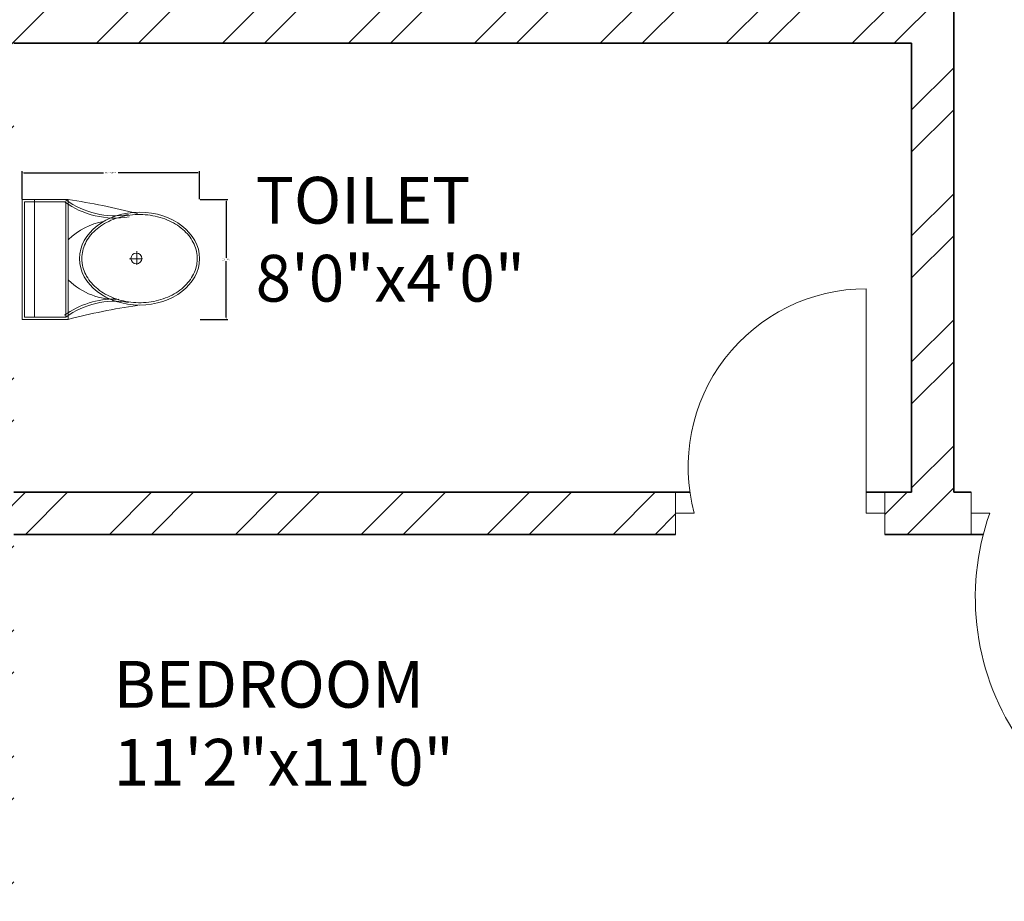
# Model space of a CAD drawing. Units: inches. Extents: x 1885 to 2748, y 783 to 2421.
# Tile 70 of 117: x 2022 to 2127, y 1979 to 2073. Entities that reach past the tile are written whole.
import ezdxf

# ---------------------------------------------------------------- set-up
doc = ezdxf.new("R2010")
doc.units = ezdxf.units.IN
for name, color, linetype, lineweight in [('A-ANNO-DIMS', 2, 'Continuous', 18), ('A-AREA-IDEN', 7, 'Continuous', 18), ('A-DOOR', 31, 'Continuous', 18), ('A-FLOR-FIXT', 8, 'Continuous', 18), ('A-WALL', 7, 'Continuous', 35)]:
    doc.layers.add(name, color=color, linetype=linetype, lineweight=lineweight)
doc.layers.add('A-WALL-PATT', color=85, linetype='Continuous', lineweight=13, true_color=0x58ba48)
doc.styles.get("Standard").update_dxf_attribs({"font": 'arial.ttf'})
doc.dimstyles.get("Standard").update_dxf_attribs({"dimtxt": 0.18, "dimasz": 0.18, "dimexe": 0.18, "dimexo": 0.0625, "dimgap": 0.09, "dimtad": 0, "dimtih": 1, "dimtoh": 1, "dimdec": 4, "dimzin": 0, "dimdsep": 46, "dimtxsty": 'Standard', "dimcen": 0.09, "dimadec": 0, "dimazin": 0, "dimtfac": 1, "dimtdec": 4, "dimtofl": 0, "dimtmove": 0, "dimatfit": 3, "dimfxl": 1, "dimtolj": 1, "dimtzin": 0, "dimarcsym": 0})

# ---------------------------------------------------------------- blocks, each defined once
blk = doc.blocks.new('A$C31115884')
for p, q in [((257.5, 466.4), (257.5, 523.2)), ((283.1, 497.7), (223.4, 497.7)), ((0, 200), (0, 0)), ((520, 200), (0, 200)), ((10, 190), (10, 10)), ((510, 190), (10, 190)), ((510, 10), (510, 190)), ((520, 0), (520, 200)), ((510, 54.5), (0, 54.5)), ((10, 10), (510, 10)), ((0, 0), (520, 0))]:
    blk.add_line(p, q)
blk.add_circle((255.6, 496.4), 23.6)
for centre, radius, start, end in [((2777.7, -204.6), 2807, 165.4549, 171.7133), ((3237, 905), 2807, 188.2867, 194.5451), ((-294.5, 403.3), 364.7, 324.2091, 9.3499), ((-294.5, 403.3), 374.7, 324.2091, 9.3499), ((805.8, 403.3), 364.7, 170.6501, 215.7909), ((139.5, 406.2), 293.5, 315.8436, 2.6563), ((805.8, 403.3), 374.7, 179.2036, 215.7909), ((383.6, 406.2), 293.5, 190.2774, 224.1564)]:
    blk.add_arc(centre, radius, start, end)
blk.add_ellipse((256.2, 509.9), major_axis=(0, -260.7), ratio=0.772727)
blk.add_open_spline([(256.2, 259.2), (263.1, 259.2), (270, 259.7), (287.8, 262.3), (298.7, 265.1), (319.9, 273.1), (330.2, 278.4), (350.1, 291.1), (359.7, 298.7), (377.7, 315.9), (386.2, 325.5), (401.7, 346.6), (408.8, 358.1), (421.3, 382.5), (426.8, 395.5), (435.9, 422.4), (439.5, 436.4), (444.8, 465.1), (446.5, 479.7), (447.9, 509.2), (447.6, 524), (445, 553.3), (442.7, 567.8), (436.3, 596), (432.1, 609.7), (421.9, 636), (416, 648.6), (402.5, 672.1), (395, 683), (378.6, 703), (369.8, 712.1), (351.1, 728), (341.3, 734.8), (320.9, 746.2), (310.4, 750.7), (288.9, 757.3), (278, 759.4), (256, 761), (245, 760.6), (223.1, 757.2), (212.3, 754.3), (191.1, 746.1), (180.8, 740.7), (160.9, 727.8), (151.4, 720.1), (133.5, 702.7), (125.1, 693), (109.6, 671.7), (102.6, 660.2), (90.2, 635.7), (84.9, 622.7), (76, 595.6), (72.4, 581.6), (67.2, 552.9), (65.6, 538.2), (64.4, 508.8), (64.8, 494), (67.5, 464.7), (69.9, 450.2), (76.6, 422), (80.8, 408.3), (91.1, 382.2), (97.2, 369.7), (110.8, 346.3), (118.4, 335.4), (134.8, 315.6), (143.7, 306.7), (162.4, 290.9), (172.3, 284.2), (192.8, 273), (203.3, 268.6), (224.8, 262.2), (235.8, 260.2), (249.9, 259.3), (253, 259.2), (256.2, 259.2)], degree=3, knots=[0, 0, 0, 0, 0.110105, 0.110105, 0.285049, 0.285049, 0.459994, 0.459994, 0.634938, 0.634938, 0.809882, 0.809882, 0.984827, 0.984827, 1.159771, 1.159771, 1.334715, 1.334715, 1.50966, 1.50966, 1.684604, 1.684604, 1.859549, 1.859549, 2.034493, 2.034493, 2.209437, 2.209437, 2.384382, 2.384382, 2.559326, 2.559326, 2.73427, 2.73427, 2.909215, 2.909215, 3.084159, 3.084159, 3.259103, 3.259103, 3.434048, 3.434048, 3.608992, 3.608992, 3.783936, 3.783936, 3.958881, 3.958881, 4.133825, 4.133825, 4.30877, 4.30877, 4.483714, 4.483714, 4.658658, 4.658658, 4.833603, 4.833603, 5.008547, 5.008547, 5.183491, 5.183491, 5.358436, 5.358436, 5.53338, 5.53338, 5.708324, 5.708324, 5.883269, 5.883269, 6.058213, 6.058213, 6.233158, 6.233158, 6.283185, 6.283185, 6.283185, 6.283185])
blk = doc.blocks.new('*D29')
at = {"layer": 'A-ANNO-DIMS', "color": 0, "lineweight": -2, "transparency": 16777216}
for p, q in [((2022.15, 2053.85), (2022.15, 2056.82)), ((2022.33, 2056.64), (2030.86, 2056.64)), ((2040.95, 2056.64), (2032.42, 2056.64)), ((2041.13, 2053.85), (2041.13, 2056.82))]:
    blk.add_line(p, q, dxfattribs=at)
at = {"layer": 'A-ANNO-DIMS', "color": 0, "transparency": 16777216}
for points in [[(2022.33, 2056.67), (2022.33, 2056.61), (2022.15, 2056.64)], [(2040.95, 2056.67), (2040.95, 2056.61), (2041.13, 2056.64)]]:
    blk.add_solid(points, dxfattribs=at)
at = {"layer": 'Defpoints', "color": 0, "transparency": 16777216}
for p in [(2041.13, 2056.64), (2022.15, 2053.79), (2041.13, 2053.79)]:
    blk.add_point(p, dxfattribs=at)
at = {"layer": 'A-ANNO-DIMS', "color": 0, "transparency": 16777216, "insert": (2031.64, 2056.64), "char_height": 0.18, "attachment_point": 5}
blk.add_mtext('\\A1;WC 19 TYP.', dxfattribs=at)
blk = doc.blocks.new('*D30')
at = {"layer": 'A-ANNO-DIMS', "color": 0, "lineweight": -2, "transparency": 16777216}
for p, q in [((2041.19, 2053.79), (2044.15, 2053.79)), ((2043.97, 2053.61), (2043.97, 2047.57)), ((2043.97, 2041.17), (2043.97, 2047.21)), ((2041.19, 2040.99), (2044.15, 2040.99))]:
    blk.add_line(p, q, dxfattribs=at)
at = {"layer": 'A-ANNO-DIMS', "color": 0, "transparency": 16777216}
for points in [[(2043.94, 2053.61), (2044, 2053.61), (2043.97, 2053.79)], [(2043.94, 2041.17), (2044, 2041.17), (2043.97, 2040.99)]]:
    blk.add_solid(points, dxfattribs=at)
at = {"layer": 'Defpoints', "color": 0, "transparency": 16777216}
for p in [(2041.13, 2053.79), (2041.13, 2040.99), (2043.97, 2040.99)]:
    blk.add_point(p, dxfattribs=at)
at = {"layer": 'A-ANNO-DIMS', "color": 0, "transparency": 16777216, "insert": (2043.97, 2047.39), "char_height": 0.18, "attachment_point": 5}
blk.add_mtext('\\A1;13 TYP.', dxfattribs=at)

msp = doc.modelspace()

# ---------------------------------------------------------------- hatches: boundary and pattern name
at = {"layer": 'A-WALL-PATT'}
h = msp.add_hatch(dxfattribs=at)
h.set_pattern_fill('ANSI32', color=256)
h.paths.add_polyline_path([(2007.77, 2318.01), (1980.77, 2318.01), (1980.77, 2281.22), (1985.27, 2281.22), (1985.27, 2313.51), (2007.77, 2313.51), (2007.77, 2315.76)])
h.paths.add_polyline_path([(2094.32, 2318.01), (2067.77, 2318.01), (2067.77, 2313.51), (2094.32, 2313.51), (2094.32, 2315.76)])
h.paths.add_polyline_path([(2131.37, 2315.76), (2131.37, 2318.01), (2131.19, 2318.01), (2112.61, 2318.01), (2112.61, 2313.51), (2117.27, 2313.51), (2117.27, 2255.2), (2121.77, 2255.2), (2121.77, 2313.51), (2131.37, 2313.51)])
h.paths.add_polyline_path([(2190.51, 2318.01), (2155.37, 2318.01), (2155.37, 2313.51), (2169.77, 2313.51), (2169.77, 2229.51), (2121.77, 2229.51), (2121.77, 2233.45), (2119.52, 2233.45), (2117.27, 2233.45), (2117.27, 2201.1), (2121.77, 2201.1), (2121.77, 2225.01), (2169.77, 2225.01), (2169.77, 2165.01), (2306.27, 2165.01), (2306.27, 2066.01), (2310.77, 2066.01), (2344.27, 2066.01), (2486.27, 2066.01), (2486.27, 1886.01), (2483.02, 1886.01), (2483.02, 1881.51), (2486.27, 1881.51), (2486.27, 1880.68), (2490.77, 1880.68), (2490.77, 2070.51), (2344.27, 2070.51), (2310.77, 2070.51), (2310.77, 2165.01), (2310.77, 2173.64), (2308.52, 2173.64), (2306.27, 2173.64), (2306.27, 2169.51), (2174.27, 2169.51), (2174.27, 2313.51), (2190.51, 2313.51), (2190.51, 2315.76)])
h.paths.add_polyline_path([(1985.27, 2221.22), (1980.77, 2221.22), (1980.77, 2165.01), (1992.77, 2165.01), (1992.77, 2141.93), (1997.27, 2141.93), (1997.27, 2165.01), (2117.27, 2165.01), (2117.27, 2163.13), (2121.77, 2163.13), (2121.77, 2172.73), (2119.52, 2172.73), (2117.27, 2172.73), (2117.27, 2169.51), (1985.27, 2169.51)])
h.paths.add_polyline_path([(1997.27, 2105.93), (1992.77, 2105.93), (1992.77, 2070.51), (2016.77, 2070.51), (2016.77, 2059.12), (2019.02, 2059.12), (2021.27, 2059.12), (2021.27, 2070.51), (2117.27, 2070.51), (2117.27, 2022.51), (2114.42, 2022.51), (2114.42, 2018.01), (2123.63, 2018.01), (2123.63, 2020.26), (2123.63, 2022.51), (2121.77, 2022.51), (2121.77, 2142.59), (2119.52, 2142.59), (2117.27, 2142.59), (2117.27, 2075.01), (1997.27, 2075.01)])
h.paths.add_polyline_path([(2092.03, 2020.26), (2092.03, 2022.51), (2021.27, 2022.51), (2021.27, 2035.12), (2016.77, 2035.12), (2016.77, 2018.01), (2016.77, 1978.78), (2021.27, 1978.78), (2021.27, 2018.01), (2092.03, 2018.01)])
h.paths.add_polyline_path([(2260.94, 2022.51), (2153.1, 2022.51), (2153.1, 2020.26), (2153.1, 2018.01), (2155.27, 2018.01), (2155.27, 1886.01), (2107.63, 1886.01), (2107.63, 1881.51), (2182.91, 1881.51), (2182.91, 1883.76), (2182.91, 1886.01), (2159.77, 1886.01), (2159.77, 2018.01), (2260.94, 2018.01), (2260.94, 2020.26)])
h.paths.add_polyline_path([(2047.63, 1883.76), (2047.63, 1886.01), (2021.27, 1886.01), (2021.27, 1918.78), (2019.02, 1918.78), (2016.77, 1918.78), (2016.77, 1881.51), (2047.63, 1881.51)])
h.paths.add_polyline_path([(2306.36, 1883.76), (2306.36, 1886.01), (2296.27, 1886.01), (2296.27, 1982.01), (2316.54, 1982.01), (2316.54, 1984.26), (2316.54, 1986.51), (2296.27, 1986.51), (2296.27, 2022.51), (2289.28, 2022.51), (2289.28, 2018.01), (2291.77, 2018.01), (2291.77, 1886.01), (2242.91, 1886.01), (2242.91, 1881.51), (2306.36, 1881.51)], flags=17)
h.paths.add_polyline_path([(1985.27, 1843.01), (2021.6, 1843.01), (2021.53, 1845.44), (2021.48, 1847.51), (1980.77, 1847.51), (1980.77, 1809.45), (1985.27, 1809.45)])
h.paths.add_polyline_path([(2131.48, 1845.26), (2131.48, 1847.51), (2081.53, 1847.51), (2081.53, 1843.01), (2117.27, 1843.01), (2117.27, 1784.15), (2119.52, 1784.15), (2121.77, 1784.15), (2121.77, 1843.01), (2131.48, 1843.01)])
h.paths.add_polyline_path([(2203.89, 1847.51), (2155.48, 1847.51), (2155.48, 1843.01), (2169.77, 1843.01), (2169.77, 1759.01), (2121.77, 1759.01), (2121.77, 1761.46), (2117.27, 1761.46), (2117.27, 1730.43), (2121.77, 1730.43), (2121.77, 1754.51), (2177.42, 1754.51), (2177.42, 1756.76), (2177.42, 1759.01), (2174.27, 1759.01), (2174.27, 1843.01), (2203.89, 1843.01)])
h.paths.add_polyline_path([(2335.55, 1845.26), (2335.55, 1847.51), (2239.89, 1847.51), (2239.89, 1843.01), (2306.27, 1843.01), (2306.27, 1759.01), (2199.49, 1759.01), (2199.49, 1754.51), (2310.77, 1754.51), (2310.77, 1843.01), (2335.55, 1843.01)])
h.paths.add_polyline_path([(2348.77, 2022.51), (2344.27, 2022.51), (2344.27, 1986.51), (2341.68, 1986.51), (2341.68, 1982.01), (2344.27, 1982.01), (2344.27, 1886.01), (2330.36, 1886.01), (2330.36, 1881.51), (2361.63, 1881.51), (2361.63, 1883.76), (2361.63, 1886.01), (2348.77, 1886.01)], flags=17)
h.paths.add_polyline_path([(2283.25, 2315.76), (2283.25, 2318.01), (2238.51, 2318.01), (2238.51, 2313.51), (2283.25, 2313.51)], flags=17)
h.paths.add_polyline_path([(2363.27, 2348.01), (2388.68, 2348.01), (2388.68, 2350.26), (2388.68, 2352.51), (2358.77, 2352.51), (2358.77, 2348.01), (2358.77, 2318.01), (2344.48, 2318.01), (2344.48, 2313.51), (2358.77, 2313.51), (2358.77, 2229.51), (2310.77, 2229.51), (2310.77, 2231.95), (2306.27, 2231.95), (2306.27, 2205.61), (2310.77, 2205.61), (2310.77, 2225.01), (2358.77, 2225.01), (2358.77, 2211.51), (2452.33, 2211.51), (2452.33, 2213.76), (2452.33, 2216.01), (2363.27, 2216.01), (2363.27, 2318.01)])
h.paths.add_polyline_path([(2310.77, 2313.51), (2320.48, 2313.51), (2320.48, 2315.76), (2320.48, 2318.01), (2302.73, 2318.01), (2302.73, 2313.51), (2306.27, 2313.51), (2306.27, 2251.08), (2310.77, 2251.08)], flags=17)
h.paths.add_polyline_path([(2490.77, 2352.51), (2486.27, 2352.51), (2448.68, 2352.51), (2448.68, 2348.01), (2486.27, 2348.01), (2486.27, 2318.01), (2486.27, 2216.01), (2481.78, 2216.01), (2481.78, 2211.51), (2486.27, 2211.51), (2486.27, 2165.01), (2493.29, 2165.01), (2493.29, 2167.26), (2493.29, 2169.51), (2490.77, 2169.51), (2490.77, 2313.51), (2494.43, 2313.51), (2494.43, 2318.01), (2490.77, 2318.01)])
h.paths.add_polyline_path([(2534.65, 2318.01), (2515.69, 2318.01), (2515.69, 2313.51), (2534.65, 2313.51), (2534.65, 2315.76)])
h.paths.add_polyline_path([(2618.27, 2318.01), (2594.65, 2318.01), (2594.65, 2313.51), (2613.77, 2313.51), (2613.77, 2281.71), (2618.27, 2281.71)])
h.paths.add_polyline_path([(2618.27, 2221.71), (2613.77, 2221.71), (2613.77, 2169.51), (2554.02, 2169.51), (2554.02, 2165.01), (2613.77, 2165.01), (2613.77, 2152.88), (2618.27, 2152.88)])
h.paths.add_polyline_path([(2618.27, 2128.88), (2616.02, 2128.88), (2613.77, 2128.88), (2613.77, 2117.01), (2529.77, 2117.01), (2529.77, 2165.01), (2532.85, 2165.01), (2532.85, 2169.51), (2522.87, 2169.51), (2522.87, 2165.01), (2525.27, 2165.01), (2525.27, 2117.01), (2525.27, 2112.51), (2525.27, 2108.58), (2529.77, 2108.58), (2529.77, 2112.51), (2613.77, 2112.51), (2613.77, 2080.19), (2618.27, 2080.19)])
h.paths.add_polyline_path([(2618.27, 2044.19), (2616.02, 2044.19), (2613.77, 2044.19), (2613.77, 2015.51), (2529.77, 2015.51), (2529.77, 2088.58), (2527.52, 2088.58), (2525.27, 2088.58), (2525.27, 2011.01), (2613.77, 2011.01), (2613.77, 1956.75), (2618.27, 1956.75)])
h.paths.add_polyline_path([(2618.27, 1881.51), (2618.27, 1896.75), (2613.77, 1896.75), (2613.77, 1881.51), (2613.77, 1847.51), (2592.71, 1847.51), (2592.71, 1843.01), (2613.77, 1843.01), (2613.77, 1765.01), (2613.77, 1760.51), (2609.62, 1760.51), (2609.62, 1756.01), (2613.77, 1756.01), (2613.77, 1660.01), (2608.54, 1660.01), (2608.54, 1655.51), (2613.77, 1655.51), (2613.77, 1508.16), (2618.27, 1508.16)])
h.paths.add_polyline_path([(2565.77, 1843.01), (2569, 1843.01), (2569, 1847.51), (2490.77, 1847.51), (2490.77, 1849.7), (2488.52, 1849.7), (2486.27, 1849.7), (2486.27, 1847.51), (2477.27, 1847.51), (2477.27, 1838.51), (2477.27, 1821.49), (2486.27, 1821.49), (2486.27, 1838.51), (2561.27, 1838.51), (2561.27, 1765.01), (2486.27, 1765.01), (2486.27, 1786.16), (2477.27, 1786.16), (2477.27, 1765.01), (2477.27, 1756.01), (2486.27, 1756.01), (2565.77, 1756.01), (2585.62, 1756.01), (2585.62, 1758.26), (2585.62, 1760.51), (2565.77, 1760.51), (2565.77, 1765.01)])
h.paths.add_polyline_path([(2486.27, 1651.01), (2561.27, 1651.01), (2561.27, 1567.01), (2486.27, 1567.01), (2486.27, 1591.32), (2477.27, 1591.32), (2477.27, 1567.01), (2477.27, 1558.01), (2477.27, 1555.44), (2481.77, 1555.44), (2481.77, 1558.01), (2568.65, 1558.01), (2568.65, 1560.26), (2568.65, 1562.51), (2565.77, 1562.51), (2565.77, 1655.51), (2584.54, 1655.51), (2584.54, 1657.76), (2584.54, 1660.01), (2565.77, 1660.01), (2486.27, 1660.01), (2477.27, 1660.01), (2477.27, 1651.01), (2477.27, 1632.99), (2486.27, 1632.99)])
h.paths.add_polyline_path([(2449.97, 1883.76), (2449.97, 1886.01), (2421.63, 1886.01), (2421.63, 1881.51), (2449.97, 1881.51)], flags=17)
h.paths.add_polyline_path([(2447.27, 1847.51), (2395.55, 1847.51), (2395.55, 1843.01), (2442.77, 1843.01), (2442.77, 1809.27), (2447.27, 1809.27)])
h.paths.add_polyline_path([(1985.27, 1749.45), (1980.77, 1749.45), (1980.77, 1694.5), (1985.27, 1694.5), (1985.27, 1694.51), (1986.9, 1694.51), (1986.9, 1697.78), (1986.9, 1699.01), (1985.27, 1699.01)])
h.paths.add_polyline_path([(2152.77, 1699.01), (2121.77, 1699.01), (2121.77, 1703.67), (2119.52, 1703.67), (2117.27, 1703.67), (2117.27, 1699.01), (2009.22, 1699.01), (2009.22, 1694.51), (2148.27, 1694.51), (2148.27, 1692.63), (2152.77, 1692.63)])
h.paths.add_polyline_path([(2016.27, 1694.51), (2011.77, 1694.51), (2011.77, 1558.01), (2040.81, 1558.01), (2040.81, 1560.26), (2040.81, 1562.51), (2016.27, 1562.51)])
h.paths.add_polyline_path([(2152.77, 1663.02), (2150.52, 1663.02), (2148.27, 1663.02), (2148.27, 1562.51), (2100.81, 1562.51), (2100.81, 1558.01), (2165.12, 1558.01), (2165.12, 1560.26), (2165.12, 1562.51), (2152.77, 1562.51), (2152.77, 1610.51), (2224.77, 1610.51), (2224.77, 1607.99), (2229.27, 1607.99), (2229.27, 1615.01), (2152.77, 1615.01)])
h.paths.add_polyline_path([(2238.61, 1560.26), (2238.61, 1562.51), (2229.27, 1562.51), (2229.27, 1588.76), (2227.02, 1588.76), (2224.77, 1588.77), (2224.77, 1562.51), (2189.12, 1562.51), (2189.12, 1558.01), (2238.61, 1558.01)])
h.paths.add_polyline_path([(2336.02, 1560.26), (2336.02, 1562.51), (2310.77, 1562.51), (2310.77, 1656.35), (2308.52, 1656.35), (2306.27, 1656.35), (2306.27, 1562.51), (2286.61, 1562.51), (2286.61, 1558.01), (2336.02, 1558.01)])
h.paths.add_polyline_path([(2447.27, 1690.97), (2445.02, 1690.97), (2442.77, 1690.97), (2442.77, 1687.01), (2306.27, 1687.01), (2306.27, 1680.75), (2310.77, 1680.75), (2310.77, 1682.51), (2442.77, 1682.51), (2442.77, 1562.51), (2396.02, 1562.51), (2396.02, 1558.01), (2447.27, 1558.01)])
h.paths.add_polyline_path([(2447.27, 1749.27), (2445.02, 1749.27), (2442.77, 1749.27), (2442.77, 1717.23), (2447.27, 1717.23)])
h.paths.add_polyline_path([(2044.67, 1521.76), (2044.67, 1524.01), (2007.27, 1524.01), (2007.27, 1503.49), (2009.52, 1503.49), (2011.77, 1503.49), (2011.77, 1519.51), (2044.67, 1519.51)])
h.paths.add_polyline_path([(2177.97, 1521.76), (2177.97, 1524.01), (2104.67, 1524.01), (2104.67, 1519.51), (2145.77, 1519.51), (2145.77, 1387.51), (2143.37, 1387.51), (2143.37, 1383.01), (2251.59, 1383.01), (2251.59, 1385.26), (2251.59, 1387.51), (2150.27, 1387.51), (2150.27, 1519.51), (2177.97, 1519.51)])
h.paths.add_polyline_path([(2298.7, 1524.01), (2237.97, 1524.01), (2237.97, 1519.51), (2282.27, 1519.51), (2282.27, 1387.51), (2279.68, 1387.51), (2279.68, 1383.01), (2286.77, 1383.01), (2286.77, 1419.01), (2312.45, 1419.01), (2312.45, 1421.26), (2312.45, 1423.51), (2286.77, 1423.51), (2286.77, 1519.51), (2298.7, 1519.51), (2298.7, 1521.72)], flags=17)
h.paths.add_polyline_path([(2361.9, 1521.76), (2361.9, 1524.01), (2322.7, 1524.01), (2322.7, 1519.51), (2334.77, 1519.51), (2334.77, 1423.51), (2331.93, 1423.51), (2331.93, 1419.01), (2334.77, 1419.01), (2334.77, 1387.51), (2334.77, 1383.23), (2339.27, 1383.23), (2339.27, 1387.51), (2339.27, 1519.51), (2361.9, 1519.51)], flags=17)
h.paths.add_polyline_path([(2447.27, 1521.76), (2447.27, 1524.01), (2421.9, 1524.01), (2421.9, 1519.51), (2447.27, 1519.51)], flags=17)
h.paths.add_polyline_path([(2481.77, 1529.6), (2479.52, 1529.6), (2477.27, 1529.6), (2477.27, 1524.01), (2474.49, 1524.01), (2474.49, 1519.51), (2477.27, 1519.51), (2477.27, 1334.51), (2296.77, 1334.51), (2296.77, 1240.51), (2160.27, 1240.51), (2160.27, 1180.51), (2112.27, 1180.51), (2112.27, 1207.69), (2110.02, 1207.69), (2107.77, 1207.69), (2107.77, 1171.61), (2112.27, 1171.61), (2112.27, 1176.01), (2160.27, 1176.01), (2160.27, 1092.01), (2144.22, 1092.01), (2144.22, 1087.51), (2189.5, 1087.51), (2189.5, 1089.76), (2189.5, 1092.01), (2164.77, 1092.01), (2164.77, 1236.01), (2296.77, 1236.01), (2296.77, 1231.91), (2301.27, 1231.91), (2301.27, 1330.01), (2481.77, 1330.01), (2481.77, 1387.51)])
h.paths.add_polyline_path([(2618.27, 1448.16), (2613.77, 1448.16), (2613.77, 1382.51), (2529.77, 1382.51), (2525.27, 1382.51), (2525.27, 1307.06), (2529.77, 1307.06), (2529.77, 1378.01), (2613.77, 1378.01), (2613.77, 1354.99), (2618.27, 1354.99)])
h.paths.add_polyline_path([(2618.27, 1318.99), (2613.77, 1318.99), (2613.77, 1281.01), (2529.77, 1281.01), (2529.77, 1283.79), (2527.52, 1283.79), (2525.27, 1283.79), (2525.27, 1228.51), (2516.79, 1228.51), (2516.79, 1224.01), (2533.48, 1224.01), (2533.48, 1226.26), (2533.48, 1228.51), (2529.77, 1228.51), (2529.77, 1276.51), (2613.77, 1276.51), (2613.77, 1266.02), (2618.27, 1266.02)])
h.paths.add_polyline_path([(2618.27, 1134.96), (2613.77, 1134.96), (2613.77, 1092.01), (2594.54, 1092.01), (2594.54, 1087.51), (2618.27, 1087.51)])
h.paths.add_polyline_path([(2534.54, 1092.01), (2509.77, 1092.01), (2509.77, 1087.51), (2534.54, 1087.51), (2534.54, 1089.76)])
h.paths.add_polyline_path([(2481.27, 1224.01), (2484.12, 1224.01), (2484.12, 1226.26), (2484.12, 1228.51), (2476.77, 1228.51), (2476.77, 1198.51), (2471.61, 1198.51), (2471.61, 1194.01), (2476.77, 1194.01), (2476.77, 1062.01), (2436.89, 1062.01), (2436.89, 1057.51), (2476.77, 1057.51), (2481.27, 1057.51), (2481.27, 1062.01), (2481.27, 1087.51), (2485.35, 1087.51), (2485.35, 1089.76), (2485.35, 1092.01), (2481.27, 1092.01), (2481.27, 1117.51)])
h.paths.add_polyline_path([(2439.9, 1198.51), (2349.27, 1198.51), (2349.27, 1194.01), (2349.27, 1180.51), (2301.27, 1180.51), (2301.27, 1201.9), (2299.02, 1201.9), (2296.77, 1201.9), (2296.77, 1172.34), (2299.02, 1172.34), (2301.27, 1172.34), (2301.27, 1176.01), (2349.27, 1176.01), (2349.27, 1092.01), (2334.45, 1092.01), (2334.45, 1087.51), (2349.27, 1087.51), (2349.27, 1057.51), (2353.77, 1057.51), (2376.89, 1057.51), (2376.89, 1059.76), (2376.89, 1062.01), (2353.77, 1062.01), (2353.77, 1087.51), (2353.77, 1180.51), (2353.77, 1194.01), (2439.9, 1194.01), (2439.9, 1196.26)])
h.paths.add_polyline_path([(2270.6, 1089.76), (2270.6, 1092.01), (2249.5, 1092.01), (2249.5, 1087.51), (2270.6, 1087.51)], flags=17)
h.paths.add_polyline_path([(2310.45, 1092.01), (2301.27, 1092.01), (2301.27, 1153.29), (2296.77, 1153.29), (2296.77, 1092.01), (2293.79, 1092.01), (2293.79, 1087.51), (2310.45, 1087.51), (2310.45, 1089.76)], flags=17)
h.paths.add_polyline_path([(2112.27, 1150.33), (2110.02, 1150.33), (2107.77, 1150.33), (2107.77, 1092.01), (2104.47, 1092.01), (2104.47, 1087.51), (2120.22, 1087.51), (2120.22, 1089.76), (2120.22, 1092.01), (2112.27, 1092.01)])
h.paths.add_polyline_path([(2082.17, 1092.01), (2058.14, 1092.01), (2058.14, 1087.51), (2082.17, 1087.51), (2082.17, 1089.76)])
h.paths.add_polyline_path([(1975.77, 1145.64), (1971.27, 1145.64), (1971.27, 1087.51), (1980.77, 1087.51), (1998.14, 1087.51), (1998.14, 1089.76), (1998.14, 1092.01), (1985.27, 1092.01), (1975.77, 1092.01)])
h.paths.add_polyline_path([(2112.27, 1244.38), (2110.02, 1244.38), (2107.77, 1244.38), (2107.77, 1240.51), (1992.27, 1240.51), (1992.27, 1271.01), (1987.77, 1271.01), (1987.77, 1240.51), (1980.77, 1240.51), (1975.77, 1240.51), (1971.27, 1240.51), (1971.27, 1205.64), (1975.77, 1205.64), (1975.77, 1236.01), (2107.77, 1236.01), (2107.77, 1233.44), (2112.27, 1233.44), (2112.27, 1236.01)])
h.paths.add_polyline_path([(2112.27, 1383.01), (2114.78, 1383.01), (2114.78, 1385.26), (2114.78, 1387.51), (2102.48, 1387.51), (2102.48, 1383.01), (2107.77, 1383.01), (2107.77, 1335.01), (2011.77, 1335.01), (2011.77, 1349.94), (2007.27, 1349.94), (2007.27, 1335.01), (1987.77, 1335.01), (1987.77, 1330.51), (1987.77, 1307.01), (1992.27, 1307.01), (1992.27, 1330.51), (2007.27, 1330.51), (2107.77, 1330.51), (2107.77, 1264.71), (2112.27, 1264.71)])
h.paths.add_polyline_path([(2077.86, 1387.51), (2011.77, 1387.51), (2011.77, 1390.04), (2009.52, 1390.04), (2007.27, 1390.04), (2007.27, 1373.94), (2011.77, 1373.94), (2011.77, 1383.01), (2077.86, 1383.01)])
h.paths.add_polyline_path([(2011.77, 1443.49), (2007.27, 1443.49), (2007.27, 1410.25), (2011.77, 1410.25)])

# ---------------------------------------------------------------- linework, layer by layer
at = {"layer": 'A-DOOR'}
for p, q in [((2112.42, 2020.26), (2112.42, 2044.26)), ((2092.03, 2022.51), (2092.03, 2018.01)), ((2114.42, 2022.51), (2114.42, 2018.01)), ((2123.63, 2022.51), (2123.63, 2018.01)), ((2092.03, 2018.01), (2092.03, 2020.26)), ((2092.03, 2020.26), (2094.03, 2020.26)), ((2114.42, 2020.26), (2112.42, 2020.26)), ((2114.42, 2018.01), (2114.42, 2020.26)), ((2123.63, 2018.01), (2123.63, 2020.26)), ((2123.63, 2020.26), (2125.63, 2020.26))]:
    msp.add_line(p, q, dxfattribs=at)
for centre, radius, start, end in [((2112.42, 2025.21), 19.05, 90, 195.0668), ((2151.1, 2011.27), 27.02, 160.576, 270)]:
    msp.add_arc(centre, radius, start, end, dxfattribs=at)
at = {"layer": 'A-WALL'}
for p, q in [((2121.77, 2142.59), (2121.77, 2022.51)), ((2021.27, 2070.51), (2117.27, 2070.51)), ((2117.27, 2070.51), (2117.27, 2022.51)), ((2021.27, 2022.51), (2093.57, 2022.51)), ((2112.42, 2022.51), (2117.27, 2022.51)), ((2123.63, 2022.51), (2121.77, 2022.51)), ((2021.27, 2018.01), (2092.03, 2018.01)), ((2114.42, 2018.01), (2124.94, 2018.01))]:
    msp.add_line(p, q, dxfattribs=at)

# ---------------------------------------------------------------- block references
at = {"layer": 'A-FLOR-FIXT', "xscale": 0.0246256636748975, "yscale": 0.0246256636748975, "zscale": 0.0246256636748975, "rotation": 270}
msp.add_blockref('A$C31115884', (2022.15, 2053.79), dxfattribs=at)

# ---------------------------------------------------------------- texts
at = {"layer": 'A-AREA-IDEN', "char_height": 5, "attachment_point": 1}
for s, width, insert in [('TOILET\\P8\'0"x4\'0"', 107.8947, (2047.13, 2056.22)), ('BEDROOM\\P11\'2"x11\'0"', 111.3682, (2031.94, 2004.48))]:
    msp.add_mtext_dynamic_manual_height_columns(s, width=width, gutter_width=12.5, heights=[0], dxfattribs=dict(at, insert=insert))

# ---------------------------------------------------------------- dimensions: what is measured, and where the dimension line sits
at = {"layer": 'A-ANNO-DIMS'}
dim = msp.add_linear_dim(base=(2041.13, 2056.64), p1=(2022.15, 2053.79), p2=(2041.13, 2053.79), text='WC <> TYP.', dimstyle='Standard', override={"dimdec": 0, "dimlfac": 1, "dimrnd": 0, "dimzin": 0, "dimdsep": 46, "dimlunit": 2}, dxfattribs=at)
dim.commit()
dim.dimension.update_dxf_attribs({"geometry": '*D29', "text_midpoint": (2031.64, 2056.64)})
dim = msp.add_linear_dim(base=(2043.97, 2040.99), p1=(2041.13, 2053.79), p2=(2041.13, 2040.99), angle=270, text='<> TYP.', dimstyle='Standard', override={"dimdec": 0, "dimlfac": 1, "dimrnd": 0, "dimzin": 0, "dimdsep": 46, "dimlunit": 2}, dxfattribs=at)
dim.commit()
dim.dimension.update_dxf_attribs({"geometry": '*D30', "text_midpoint": (2043.97, 2047.39)})

doc.saveas('drawing.dxf')
